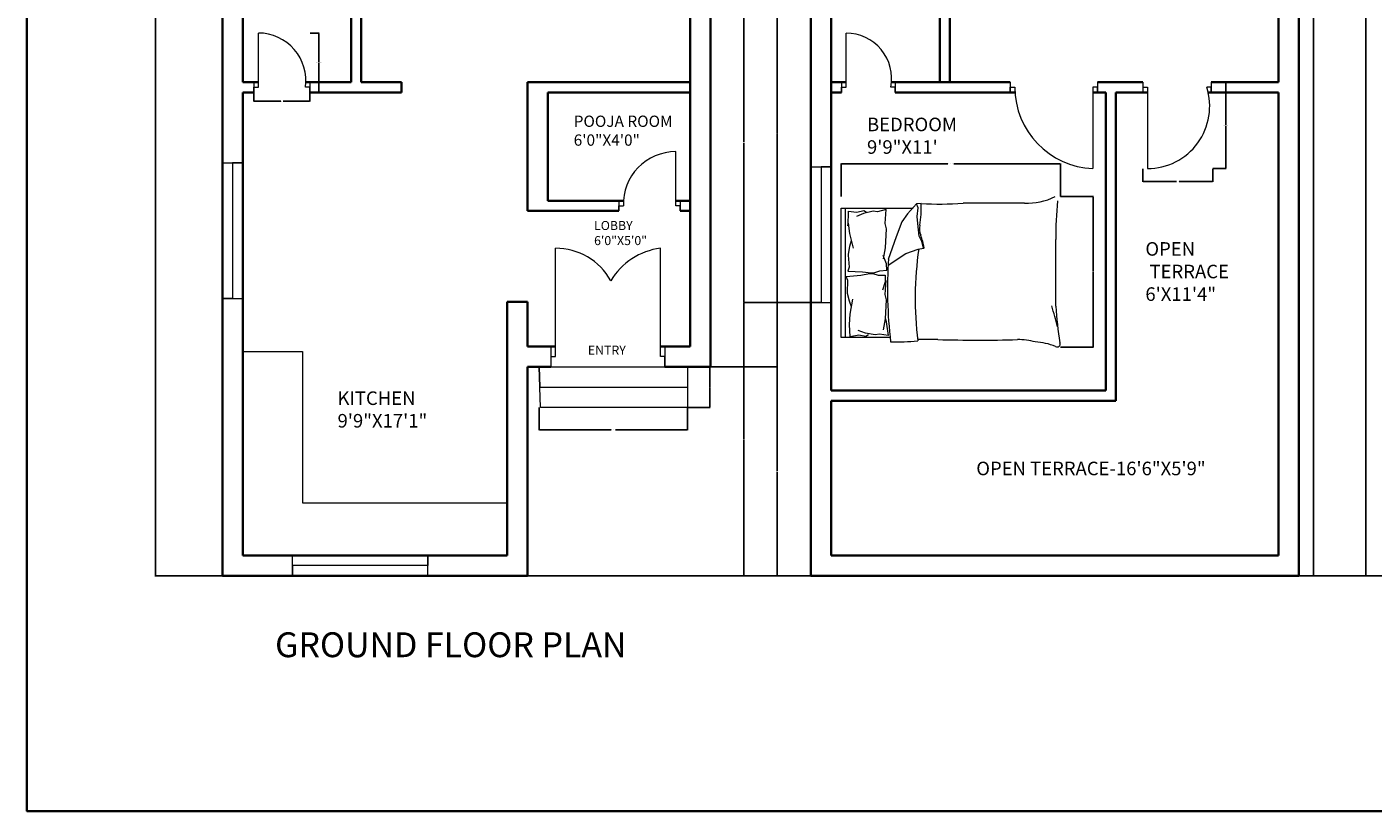
# Model space of a CAD drawing. Units: inches. Extents: x 2003 to 3241, y 1726 to 2849.
# Tile 1 of 7: x 2003 to 2599, y 1726 to 2073. Entities that reach past the tile are written whole.
import ezdxf

# ---------------------------------------------------------------- set-up
doc = ezdxf.new("R2010")
doc.units = ezdxf.units.IN
for name, color, linetype, lineweight in [('A-ANNO-DIMS', 2, 'Continuous', 18), ('A-ANNO-TEXT', 7, 'Continuous', 18), ('A-ANNO-TTLB', 7, 'Continuous', 35), ('A-AREA-IDEN', 7, 'Continuous', 18), ('A-DOOR', 3, 'Continuous', 18), ('A-FLOR-FIXT', 9, 'Continuous', 18), ('A-FLOR-STRS', 7, 'Continuous', 18), ('A-FURN', 8, 'Continuous', 13), ('A-GLAZ', 4, 'Continuous', 18), ('A-WALL', 7, 'Continuous', 35)]:
    doc.layers.add(name, color=color, linetype=linetype, lineweight=lineweight)
doc.styles.get("Standard").update_dxf_attribs({"font": 'arial.ttf'})
doc.dimstyles.get("Standard").update_dxf_attribs({"dimtxt": 0.18, "dimasz": 0.18, "dimexe": 0.18, "dimexo": 0.0625, "dimgap": 0.09, "dimtad": 0, "dimtih": 1, "dimtoh": 1, "dimdec": 4, "dimzin": 0, "dimdsep": 46, "dimtxsty": 'Standard', "dimcen": 0.09, "dimadec": 0, "dimazin": 0, "dimtfac": 1, "dimtdec": 4, "dimtofl": 0, "dimtmove": 0, "dimatfit": 3, "dimfxl": 1, "dimtolj": 1, "dimtzin": 0, "dimarcsym": 0})

# ---------------------------------------------------------------- blocks, each defined once
blk = doc.blocks.new('WIN-60-1')
for p, q in [((0, 60), (9, 60)), ((9, 60), (4.5, 60)), ((4.5, 60), (4.5, 0)), ((4.5, 0), (0, 0)), ((0, 0), (9, 0))]:
    blk.add_line(p, q)
blk = doc.blocks.new('DOOR-ENTRY-PAIR')
for p, q in [((2, 4.5), (2, 52.5)), ((48.48, 4.5), (48.48, 52.5)), ((0, 9), (0, 0)), ((50.48, 9), (50.48, 0)), ((0, 4.5), (2, 4.5)), ((50.48, 4.5), (48.48, 4.5)), ((50.48, 0), (50.48, 4.5))]:
    blk.add_line(p, q)
for centre, radius, start, end in [((2, 24.35), 28.14, 29.23528, 90), ((52.39, 22.67), 30.08, 97.45976, 149.14255)]:
    blk.add_arc(centre, radius, start, end)
blk = doc.blocks.new('DOOR-POOJA')
for p, q in [((25.16, 2.25), (25.16, 26.25)), ((0, 4.5), (0, 0)), ((0, 0), (0, 2.25)), ((0, 2.25), (2, 2.25)), ((27.16, 2.25), (25.16, 2.25)), ((27.16, 4.5), (27.16, 0)), ((27.16, 0), (27.16, 2.25))]:
    blk.add_line(p, q)
blk.add_arc((25.16, 3.08), 23.17, 90, 182.04429)
blk = doc.blocks.new('DOOR-STORE')
for p, q in [((2, 2.25), (2, 26.25)), ((0, 4.5), (0, 0)), ((0, 0), (0, 2.25)), ((0, 2.25), (2, 2.25)), ((24.85, 2.25), (22.85, 2.25)), ((24.85, 4.5), (24.85, 0)), ((24.85, 0), (24.85, 2.25))]:
    blk.add_line(p, q)
blk.add_arc((2, 5.2), 21.05, 351.95387, 90)
blk = doc.blocks.new('DOOR-TERRACE-BEDROOM')
for p, q in [((0, 38.25), (0, 33.75)), ((0, 33.75), (0, 36)), ((0, 36), (2, 36)), ((38.56, 36), (36.56, 36)), ((36.56, 36), (36.56, 0)), ((38.56, 38.25), (38.56, 33.75)), ((38.56, 33.75), (38.56, 36))]:
    blk.add_line(p, q)
blk.add_arc((38.03, 36), 36.03, 180, 267.65676)
blk = doc.blocks.new('DOOR-TERRACE')
for p, q in [((0, 38.25), (0, 33.75)), ((0, 36), (2, 36)), ((2, 36), (2, 0)), ((30.26, 36), (28.26, 36)), ((30.26, 38.25), (30.26, 33.75)), ((30.26, 33.75), (30.26, 36))]:
    blk.add_line(p, q)
blk.add_arc((2, 27.58), 27.58, 270, 17.78542)
blk = doc.blocks.new('STEPS-ENTRY')
for p, q in [((0.54, 0), (0, 18)), ((0, 18), (0.27, 9)), ((5.21, 18), (55.69, 18)), ((55.69, 18), (65.74, 18)), ((65.74, 18), (65.74, 0)), ((0.27, 9), (0.27, 9)), ((0.27, 9), (65.74, 9)), ((65.74, 0), (0.54, 0))]:
    blk.add_line(p, q)
blk = doc.blocks.new('COUNTER-KITCHEN-L')
for p, q in [((0, 67), (26.53, 67)), ((26.53, 67), (26.53, 0)), ((26.53, 0), (117, 0))]:
    blk.add_line(p, q)
blk = doc.blocks.new('BED-DOUBLE')
for p, q in [((4.17, 75.16), (4.17, 96.87)), ((4.17, 96.87), (61.46, 96.87)), ((61.46, 96.87), (61.46, 64.97)), ((4.17, 95.03), (61.46, 95.03)), ((4.67, 92.87), (9.81, 93.27)), ((4.67, 92.9), (5.36, 89.08)), ((6.06, 86.14), (7.27, 89.43)), ((9.81, 93.27), (9.93, 93.24)), ((9.93, 93.24), (14.52, 92.9)), ((14.52, 92.9), (21.1, 91.68)), ((17.81, 92.38), (20.24, 93.24)), ((20.24, 93.24), (23.7, 94.11)), ((23.7, 94.11), (24.09, 94.11)), ((24.09, 94.11), (29.42, 93.94)), ((29.42, 93.94), (31.15, 94.63)), ((31.15, 94.63), (31.84, 88.22)), ((33.54, 93.89), (33.25, 87.44)), ((35.31, 93.3), (33.54, 93.89)), ((40.62, 93.81), (35.31, 93.3)), ((41.01, 93.83), (40.62, 93.81)), ((44.52, 93.18), (41.01, 93.83)), ((50.25, 93.19), (43.75, 91.57)), ((47, 92.47), (44.52, 93.18)), ((54.8, 93.82), (50.25, 93.19)), ((60.08, 93.81), (53.6, 93.92)), ((53.6, 93.92), (54.8, 93.82)), ((59.12, 86.97), (57.7, 90.18)), ((60.08, 93.81), (59.62, 89.96)), ((59.62, 89.96), (60.34, 86.88)), ((5.36, 89.08), (4.84, 85.96)), ((4.84, 85.96), (5.54, 84.75)), ((5.36, 81.8), (6.06, 86.14)), ((31.84, 88.22), (32.54, 84.4)), ((32.54, 84.4), (32.54, 82.84)), ((33.25, 87.44), (32.79, 83.59)), ((32.79, 83.59), (32.89, 82.03)), ((60.08, 82.69), (59.12, 86.97)), ((60.34, 86.88), (59.72, 85.62)), ((5.02, 76.08), (5.71, 79.9)), ((5.71, 79.9), (5.36, 81.8)), ((7.65, 78.14), (12.48, 77.34)), ((20.89, 76.82), (23.24, 77.49)), ((23.24, 77.49), (29.39, 77)), ((28.9, 77.38), (25.13, 78.68)), ((32.54, 82.84), (31.84, 80.59)), ((31.84, 80.59), (31.84, 77.38)), ((32.89, 82.03), (33.72, 79.83)), ((33.72, 79.83), (33.93, 76.62)), ((36.87, 76.8), (40.55, 78.34)), ((39.04, 78.14), (43.87, 77.34)), ((52.28, 76.82), (54.63, 77.49)), ((54.63, 77.49), (60.78, 77)), ((59.85, 80.77), (60.08, 82.69)), ((60.78, 77), (59.85, 80.77)), ((11.13, 76.95), (5.02, 76.08)), ((12.48, 77.34), (11.13, 76.95)), ((12.48, 77.34), (20.89, 76.82)), ((31.84, 77.38), (28.9, 77.38)), ((33.93, 76.62), (36.87, 76.8)), ((36.28, 76.03), (41.3, 68.25)), ((48.73, 72.52), (38.73, 76.03)), ((43.87, 77.34), (52.28, 76.82)), ((55.41, 70.1), (48.73, 72.52)), ((41.3, 68.25), (43.34, 62.87)), ((58.94, 67.51), (55.41, 70.1)), ((63.38, 63.61), (58.94, 67.51)), ((43.34, 62.87), (43.71, 60.45)), ((43.71, 60.45), (46.68, 61.2)), ((46.68, 61.2), (49.1, 62.31)), ((49.1, 62.31), (53.18, 62.87)), ((53.18, 62.87), (57.82, 63.24)), ((57.82, 63.24), (61.54, 62.87)), ((61.54, 62.87), (63.38, 63.61)), ((63.48, 61.52), (63.38, 63.61, 4.64)), ((18.06, 1.87), (47.57, 1.87))]:
    blk.add_line(p, q)
for centre, radius, start, end in [((102.1, 72.78), 99.87, 178.72178, 185.60397), ((25.61, -121.38), 197.77, 86.08655, 96.78213), ((21.29, -90.53), 154.68, 81.78449, 96.90062), ((-200.58, 59.5), 203.94, 358.4762, 1.00819), ((43.92, 60.38), 0.221, 160.24637, 271.13765), ((37.35, 95.1), 35.55, 280.66171, 289.88058), ((52.44, 54.83), 7.46, 78.6608, 113.73842), ((61.53, 104.85), 43.38, 259.87628, 272.56571), ((218.51, 53.34), 155.25, 176.97912, 183.83645), ((581.23, 36.19), 578.22, 178.22771, 181.71854), ((-5405.34, 15.56), 5469.02, 0.00217, 0.28689), ((-32.25, 19.53), 35.53, 346.06484, 358.91125), ((91.3, 14.55), 27.65, 177.47136, 206.46809), ((-25.97, 12.62), 28.25, 337.97508, 356.652), ((1.3, 1.3), 1.31, 146.17358, 293.47814), ((25.69, -143.9), 145.97, 92.99578, 99.40907), ((-20.65, 125.3), 127.63, 283.38322, 287.70533), ((49.34, -157.62), 159.5, 84.4998, 90.63509)]:
    blk.add_arc(centre, radius, start, end)
blk = doc.blocks.new('*D26')
at = {"layer": 'A-ANNO-DIMS', "color": 0, "lineweight": -2, "transparency": 16777216}
for p, q in [((2363.72, 1998.31), (2363.72, 2012.98)), ((2363.9, 2012.8), (2410.85, 2012.8)), ((2460.54, 2012.8), (2413.58, 2012.8)), ((2460.72, 1998.31), (2460.72, 2012.98))]:
    blk.add_line(p, q, dxfattribs=at)
at = {"layer": 'A-ANNO-DIMS', "color": 0, "transparency": 16777216}
for points in [[(2363.9, 2012.83), (2363.9, 2012.77), (2363.72, 2012.8)], [(2460.54, 2012.83), (2460.54, 2012.77), (2460.72, 2012.8)]]:
    blk.add_solid(points, dxfattribs=at)
at = {"layer": 'Defpoints', "color": 0, "transparency": 16777216}
for p in [(2363.72, 2012.8), (2363.72, 1998.25), (2460.72, 1998.25)]:
    blk.add_point(p, dxfattribs=at)
at = {"layer": 'A-ANNO-DIMS', "color": 0, "transparency": 16777216, "insert": (2412.22, 2012.8), "char_height": 0.18, "attachment_point": 5}
blk.add_mtext('\\A1;DOUBLE BED 97 TYP.', dxfattribs=at)
blk = doc.blocks.new('*D27')
at = {"layer": 'A-ANNO-DIMS', "color": 0, "lineweight": -2, "transparency": 16777216}
for p, q in [((2460.78, 1998.25), (2475.44, 1998.25)), ((2475.26, 1998.07), (2475.26, 1965.1)), ((2475.26, 1931.78), (2475.26, 1964.74)), ((2460.78, 1931.6), (2475.44, 1931.6))]:
    blk.add_line(p, q, dxfattribs=at)
at = {"layer": 'A-ANNO-DIMS', "color": 0, "transparency": 16777216}
for points in [[(2475.23, 1998.07), (2475.29, 1998.07), (2475.26, 1998.25)], [(2475.23, 1931.78), (2475.29, 1931.78), (2475.26, 1931.6)]]:
    blk.add_solid(points, dxfattribs=at)
at = {"layer": 'Defpoints', "color": 0, "transparency": 16777216}
for p in [(2460.72, 1998.25), (2475.26, 1998.25), (2460.72, 1931.6)]:
    blk.add_point(p, dxfattribs=at)
at = {"layer": 'A-ANNO-DIMS', "color": 0, "transparency": 16777216, "insert": (2475.26, 1964.92), "char_height": 0.18, "attachment_point": 5}
blk.add_mtext('\\A1;67 TYP.', dxfattribs=at)
blk = doc.blocks.new('*D40')
at = {"layer": 'A-ANNO-DIMS', "color": 0, "lineweight": -2, "transparency": 16777216}
for p, q in [((2128.61, 2070.66), (2132.66, 2070.66)), ((2132.48, 2070.48), (2132.48, 2057.72)), ((2132.48, 2044.59), (2132.48, 2057.36)), ((2128.61, 2044.41), (2132.66, 2044.41))]:
    blk.add_line(p, q, dxfattribs=at)
at = {"layer": 'A-ANNO-DIMS', "color": 0, "transparency": 16777216}
for points in [[(2132.45, 2070.48), (2132.51, 2070.48), (2132.48, 2070.66)], [(2132.45, 2044.59), (2132.51, 2044.59), (2132.48, 2044.41)]]:
    blk.add_solid(points, dxfattribs=at)
at = {"layer": 'Defpoints', "color": 0, "transparency": 16777216}
for p in [(2128.55, 2070.66), (2132.48, 2070.66), (2128.55, 2044.41)]:
    blk.add_point(p, dxfattribs=at)
at = {"layer": 'A-ANNO-DIMS', "color": 0, "transparency": 16777216, "insert": (2132.48, 2057.54), "char_height": 0.18, "attachment_point": 5}
blk.add_mtext('\\A1;STORE DOOR 26 TYP.', dxfattribs=at)
blk = doc.blocks.new('*D41')
at = {"layer": 'A-ANNO-DIMS', "color": 0, "lineweight": -2, "transparency": 16777216}
for p, q in [((2103.7, 2044.35), (2103.7, 2040.3)), ((2128.55, 2044.35), (2128.55, 2040.3)), ((2103.88, 2040.48), (2115.59, 2040.48)), ((2128.37, 2040.48), (2116.65, 2040.48))]:
    blk.add_line(p, q, dxfattribs=at)
at = {"layer": 'A-ANNO-DIMS', "color": 0, "transparency": 16777216}
for points in [[(2103.88, 2040.51), (2103.88, 2040.45), (2103.7, 2040.48)], [(2128.37, 2040.51), (2128.37, 2040.45), (2128.55, 2040.48)]]:
    blk.add_solid(points, dxfattribs=at)
at = {"layer": 'Defpoints', "color": 0, "transparency": 16777216}
for p in [(2103.7, 2044.41), (2128.55, 2044.41), (2128.55, 2040.48)]:
    blk.add_point(p, dxfattribs=at)
at = {"layer": 'A-ANNO-DIMS', "color": 0, "transparency": 16777216, "insert": (2116.12, 2040.48), "char_height": 0.18, "attachment_point": 5}
blk.add_mtext('\\A1;25 TYP.', dxfattribs=at)
blk = doc.blocks.new('*D50')
at = {"layer": 'A-ANNO-DIMS', "color": 0, "lineweight": -2, "transparency": 16777216}
for p, q in [((2528.24, 2048.91), (2534.1, 2048.91)), ((2533.92, 2048.73), (2533.92, 2029.97)), ((2533.92, 2010.84), (2533.92, 2029.61)), ((2528.24, 2010.66), (2534.1, 2010.66))]:
    blk.add_line(p, q, dxfattribs=at)
at = {"layer": 'A-ANNO-DIMS', "color": 0, "transparency": 16777216}
for points in [[(2533.89, 2048.73), (2533.95, 2048.73), (2533.92, 2048.91)], [(2533.89, 2010.84), (2533.95, 2010.84), (2533.92, 2010.66)]]:
    blk.add_solid(points, dxfattribs=at)
at = {"layer": 'Defpoints', "color": 0, "transparency": 16777216}
for p in [(2528.18, 2048.91), (2533.92, 2048.91), (2528.18, 2010.66)]:
    blk.add_point(p, dxfattribs=at)
at = {"layer": 'A-ANNO-DIMS', "color": 0, "transparency": 16777216, "insert": (2533.92, 2029.79), "char_height": 0.18, "attachment_point": 5}
blk.add_mtext('\\A1;TERRACE DOOR 38 TYP.', dxfattribs=at)
blk = doc.blocks.new('*D51')
at = {"layer": 'A-ANNO-DIMS', "color": 0, "lineweight": -2, "transparency": 16777216}
for p, q in [((2497.23, 2010.6), (2497.23, 2004.75)), ((2528.18, 2010.6), (2528.18, 2004.75)), ((2497.41, 2004.93), (2512.18, 2004.93)), ((2528, 2004.93), (2513.23, 2004.93))]:
    blk.add_line(p, q, dxfattribs=at)
at = {"layer": 'A-ANNO-DIMS', "color": 0, "transparency": 16777216}
for points in [[(2497.41, 2004.96), (2497.41, 2004.9), (2497.23, 2004.93)], [(2528, 2004.96), (2528, 2004.9), (2528.18, 2004.93)]]:
    blk.add_solid(points, dxfattribs=at)
at = {"layer": 'Defpoints', "color": 0, "transparency": 16777216}
for p in [(2497.23, 2010.66), (2528.18, 2010.66), (2528.18, 2004.93)]:
    blk.add_point(p, dxfattribs=at)
at = {"layer": 'A-ANNO-DIMS', "color": 0, "transparency": 16777216, "insert": (2512.71, 2004.93), "char_height": 0.18, "attachment_point": 5}
blk.add_mtext('\\A1;31 TYP.', dxfattribs=at)
blk = doc.blocks.new('*D56')
at = {"layer": 'A-ANNO-DIMS', "color": 0, "lineweight": -2, "transparency": 16777216}
for p, q in [((2229.98, 1904.85), (2229.98, 1894.87)), ((2295.72, 1904.85), (2295.72, 1894.87)), ((2230.16, 1895.05), (2261.88, 1895.05)), ((2295.54, 1895.05), (2263.83, 1895.05))]:
    blk.add_line(p, q, dxfattribs=at)
at = {"layer": 'A-ANNO-DIMS', "color": 0, "transparency": 16777216}
for points in [[(2230.16, 1895.08), (2230.16, 1895.02), (2229.98, 1895.05)], [(2295.54, 1895.08), (2295.54, 1895.02), (2295.72, 1895.05)]]:
    blk.add_solid(points, dxfattribs=at)
at = {"layer": 'Defpoints', "color": 0, "transparency": 16777216}
for p in [(2229.98, 1904.91), (2295.72, 1904.91), (2295.72, 1895.05)]:
    blk.add_point(p, dxfattribs=at)
at = {"layer": 'A-ANNO-DIMS', "color": 0, "transparency": 16777216, "insert": (2262.85, 1895.05), "char_height": 0.18, "attachment_point": 5}
blk.add_mtext('\\A1;STEPS 66 TYP.', dxfattribs=at)
blk = doc.blocks.new('*D57')
at = {"layer": 'A-ANNO-DIMS', "color": 0, "lineweight": -2, "transparency": 16777216}
for p, q in [((2295.79, 1922.91), (2305.77, 1922.91)), ((2305.59, 1922.73), (2305.59, 1914.1)), ((2305.59, 1905.09), (2305.59, 1913.73)), ((2295.79, 1904.91), (2305.77, 1904.91))]:
    blk.add_line(p, q, dxfattribs=at)
at = {"layer": 'A-ANNO-DIMS', "color": 0, "transparency": 16777216}
for points in [[(2305.56, 1922.73), (2305.62, 1922.73), (2305.59, 1922.91)], [(2305.56, 1905.09), (2305.62, 1905.09), (2305.59, 1904.91)]]:
    blk.add_solid(points, dxfattribs=at)
at = {"layer": 'Defpoints', "color": 0, "transparency": 16777216}
for p in [(2295.72, 1922.91), (2305.59, 1922.91), (2295.72, 1904.91)]:
    blk.add_point(p, dxfattribs=at)
at = {"layer": 'A-ANNO-DIMS', "color": 0, "transparency": 16777216, "insert": (2305.59, 1913.91), "char_height": 0.18, "attachment_point": 5}
blk.add_mtext('\\A1;18 TYP.', dxfattribs=at)
blk = doc.blocks.new('*D65')
at = {"layer": 'A-ANNO-DIMS', "color": 0, "lineweight": -2, "transparency": 16777216}
for p, q in [((2089.72, 2369.91), (2059.95, 2369.91)), ((2060.13, 2369.73), (2060.13, 2100.35)), ((2060.13, 1830.59), (2060.13, 2099.98)), ((2089.72, 1830.41), (2059.95, 1830.41))]:
    blk.add_line(p, q, dxfattribs=at)
at = {"layer": 'A-ANNO-DIMS', "color": 0, "transparency": 16777216}
for points in [[(2060.1, 2369.73), (2060.16, 2369.73), (2060.13, 2369.91)], [(2060.1, 1830.59), (2060.16, 1830.59), (2060.13, 1830.41)]]:
    blk.add_solid(points, dxfattribs=at)
at = {"layer": 'Defpoints', "color": 0, "transparency": 16777216}
for p in [(2060.13, 2369.91), (2089.78, 2369.91), (2089.78, 1830.41)]:
    blk.add_point(p, dxfattribs=at)
at = {"layer": 'A-ANNO-DIMS', "color": 0, "transparency": 16777216, "insert": (2060.13, 2100.16), "char_height": 0.18, "attachment_point": 5}
blk.add_mtext('\\A1;539.5', dxfattribs=at)
blk = doc.blocks.new('*D66')
at = {"layer": 'A-ANNO-DIMS', "color": 0, "lineweight": -2, "transparency": 16777216}
for p, q in [((2305.84, 1922.91), (2335.61, 1922.91)), ((2335.43, 1922.73), (2335.43, 1876.85)), ((2335.43, 1830.59), (2335.43, 1876.48)), ((2224.84, 1830.41), (2335.61, 1830.41))]:
    blk.add_line(p, q, dxfattribs=at)
at = {"layer": 'A-ANNO-DIMS', "color": 0, "transparency": 16777216}
for points in [[(2335.4, 1922.73), (2335.46, 1922.73), (2335.43, 1922.91)], [(2335.4, 1830.59), (2335.46, 1830.59), (2335.43, 1830.41)]]:
    blk.add_solid(points, dxfattribs=at)
at = {"layer": 'Defpoints', "color": 0, "transparency": 16777216}
for p in [(2305.78, 1922.91), (2335.43, 1922.91), (2224.78, 1830.41)]:
    blk.add_point(p, dxfattribs=at)
at = {"layer": 'A-ANNO-DIMS', "color": 0, "transparency": 16777216, "insert": (2335.43, 1876.66), "char_height": 0.18, "attachment_point": 5}
blk.add_mtext('\\A1;92.5', dxfattribs=at)
blk = doc.blocks.new('*D67')
at = {"layer": 'A-ANNO-DIMS', "color": 0, "lineweight": -2, "transparency": 16777216}
for p, q in [((2305.84, 2129.81), (2335.61, 2129.81)), ((2335.43, 2129.63), (2335.43, 2026.55)), ((2335.43, 1923.09), (2335.43, 2026.18)), ((2305.84, 1922.91), (2335.61, 1922.91))]:
    blk.add_line(p, q, dxfattribs=at)
at = {"layer": 'A-ANNO-DIMS', "color": 0, "transparency": 16777216}
for points in [[(2335.4, 2129.63), (2335.46, 2129.63), (2335.43, 2129.81)], [(2335.4, 1923.09), (2335.46, 1923.09), (2335.43, 1922.91)]]:
    blk.add_solid(points, dxfattribs=at)
at = {"layer": 'Defpoints', "color": 0, "transparency": 16777216}
for p in [(2305.78, 2129.81), (2335.43, 2129.81), (2305.78, 1922.91)]:
    blk.add_point(p, dxfattribs=at)
at = {"layer": 'A-ANNO-DIMS', "color": 0, "transparency": 16777216, "insert": (2335.43, 2026.36), "char_height": 0.18, "attachment_point": 5}
blk.add_mtext('\\A1;206.9', dxfattribs=at)
blk = doc.blocks.new('*D71')
at = {"layer": 'A-ANNO-DIMS', "color": 0, "lineweight": -2, "transparency": 16777216}
for p, q in [((2566.36, 2369.91), (2596.13, 2369.91)), ((2595.95, 2369.73), (2595.95, 2100.35)), ((2595.95, 1830.59), (2595.95, 2099.98)), ((2566.36, 1830.41), (2596.13, 1830.41))]:
    blk.add_line(p, q, dxfattribs=at)
at = {"layer": 'A-ANNO-DIMS', "color": 0, "transparency": 16777216}
for points in [[(2595.92, 2369.73), (2595.98, 2369.73), (2595.95, 2369.91)], [(2595.92, 1830.59), (2595.98, 1830.59), (2595.95, 1830.41)]]:
    blk.add_solid(points, dxfattribs=at)
at = {"layer": 'Defpoints', "color": 0, "transparency": 16777216}
for p in [(2566.3, 2369.91), (2595.95, 2369.91), (2566.3, 1830.41)]:
    blk.add_point(p, dxfattribs=at)
at = {"layer": 'A-ANNO-DIMS', "color": 0, "transparency": 16777216, "insert": (2595.95, 2100.16), "char_height": 0.18, "attachment_point": 5}
blk.add_mtext('\\A1;539.5', dxfattribs=at)
blk = doc.blocks.new('*D72')
at = {"layer": 'A-ANNO-DIMS', "color": 0, "lineweight": -2, "transparency": 16777216}
for p, q in [((2350.24, 1951.42), (2320.47, 1951.42)), ((2320.65, 1951.24), (2320.65, 1891.09)), ((2320.65, 1830.59), (2320.65, 1890.73)), ((2350.24, 1830.41), (2320.47, 1830.41))]:
    blk.add_line(p, q, dxfattribs=at)
at = {"layer": 'A-ANNO-DIMS', "color": 0, "transparency": 16777216}
for points in [[(2320.62, 1951.24), (2320.68, 1951.24), (2320.65, 1951.42)], [(2320.62, 1830.59), (2320.68, 1830.59), (2320.65, 1830.41)]]:
    blk.add_solid(points, dxfattribs=at)
at = {"layer": 'Defpoints', "color": 0, "transparency": 16777216}
for p in [(2320.65, 1951.42), (2350.3, 1951.42), (2350.3, 1830.41)]:
    blk.add_point(p, dxfattribs=at)
at = {"layer": 'A-ANNO-DIMS', "color": 0, "transparency": 16777216, "insert": (2320.65, 1890.91), "char_height": 0.18, "attachment_point": 5}
blk.add_mtext('\\A1;121', dxfattribs=at)
blk = doc.blocks.new('*D73')
at = {"layer": 'A-ANNO-DIMS', "color": 0, "lineweight": -2, "transparency": 16777216}
for p, q in [((2350.24, 2092.82), (2320.47, 2092.82)), ((2320.65, 2092.64), (2320.65, 2022.3)), ((2320.65, 1951.6), (2320.65, 2021.94)), ((2350.24, 1951.42), (2320.47, 1951.42))]:
    blk.add_line(p, q, dxfattribs=at)
at = {"layer": 'A-ANNO-DIMS', "color": 0, "transparency": 16777216}
for points in [[(2320.62, 2092.64), (2320.68, 2092.64), (2320.65, 2092.82)], [(2320.62, 1951.6), (2320.68, 1951.6), (2320.65, 1951.42)]]:
    blk.add_solid(points, dxfattribs=at)
at = {"layer": 'Defpoints', "color": 0, "transparency": 16777216}
for p in [(2320.65, 2092.82), (2350.3, 2092.82), (2350.3, 1951.42)]:
    blk.add_point(p, dxfattribs=at)
at = {"layer": 'A-ANNO-DIMS', "color": 0, "transparency": 16777216, "insert": (2320.65, 2022.12), "char_height": 0.18, "attachment_point": 5}
blk.add_mtext('\\A1;141.4', dxfattribs=at)
blk = doc.blocks.new('*D77')
at = {"layer": 'A-ANNO-DIMS', "color": 0, "lineweight": -2, "transparency": 16777216}
for p, q in [((2632.38, 2369.91), (2572.63, 2369.91)), ((2572.81, 2369.73), (2572.81, 2100.35)), ((2572.81, 1830.59), (2572.81, 2099.98)), ((2632.38, 1830.41), (2572.63, 1830.41))]:
    blk.add_line(p, q, dxfattribs=at)
at = {"layer": 'A-ANNO-DIMS', "color": 0, "transparency": 16777216}
for points in [[(2572.78, 2369.73), (2572.84, 2369.73), (2572.81, 2369.91)], [(2572.78, 1830.59), (2572.84, 1830.59), (2572.81, 1830.41)]]:
    blk.add_solid(points, dxfattribs=at)
at = {"layer": 'Defpoints', "color": 0, "transparency": 16777216}
for p in [(2572.81, 2369.91), (2632.44, 2369.91), (2632.44, 1830.41)]:
    blk.add_point(p, dxfattribs=at)
at = {"layer": 'A-ANNO-DIMS', "color": 0, "transparency": 16777216, "insert": (2572.81, 2100.16), "char_height": 0.18, "attachment_point": 5}
blk.add_mtext('\\A1;539.5', dxfattribs=at)

msp = doc.modelspace()

# ---------------------------------------------------------------- linework, layer by layer
at = {"layer": 'A-ANNO-TTLB'}
msp.add_lwpolyline([(2003.2633, 2848.7261), (3241.1194, 2848.7261), (3241.1194, 1726.227), (2003.2633, 1726.227)], close=True, dxfattribs=at)
at = {"layer": 'A-DOOR'}
for p, q in [((2365.8505, 2046.6635), (2365.8505, 2070.6635)), ((2363.8505, 2048.9135), (2363.8505, 2044.4135)), ((2363.8505, 2044.4135), (2363.8505, 2046.6635)), ((2363.8505, 2046.6635), (2365.8505, 2046.6635)), ((2387.622, 2046.6635), (2385.622, 2046.6635)), ((2387.622, 2048.9135), (2387.622, 2044.4135)), ((2387.622, 2044.4135), (2387.622, 2046.6635))]:
    msp.add_line(p, q, dxfattribs=at)
msp.add_arc((2365.8505, 2050.5196), 20.1439, 348.9640184, 90, dxfattribs=at)
at = {"layer": 'A-WALL'}
for p, q in [((2089.7784, 2369.9135), (2089.7784, 1830.4135)), ((2305.7784, 2369.9135), (2305.7784, 1922.9135)), ((2350.3008, 2369.9135), (2350.3008, 1836.4016)), ((2566.3008, 2369.9135), (2566.3008, 1836.4016)), ((2557.3008, 2360.9135), (2557.3008, 2048.9135)), ((2151.2784, 2224.4135), (2151.2784, 2048.9135)), ((2296.7784, 2224.4135), (2296.7784, 1931.9135)), ((2359.3008, 2224.4135), (2359.3008, 1912.4135)), ((2411.8008, 2048.9135), (2411.8008, 2224.4135)), ((2098.7784, 2135.9135), (2098.7784, 2048.9135)), ((2146.7784, 2135.9135), (2146.7784, 2048.9135)), ((2407.3008, 2135.9135), (2407.3008, 2048.9135)), ((2098.7784, 2048.9135), (2105.7015, 2048.9135)), ((2098.7784, 2044.4135), (2103.7015, 2044.4135)), ((2098.7784, 2044.4135), (2098.7784, 1839.4135)), ((2126.7431, 2048.9135), (2146.7784, 2048.9135)), ((2128.5474, 2044.4135), (2151.2784, 2044.4135)), ((2151.2784, 2048.9135), (2169.1304, 2048.9135)), ((2151.2784, 2044.4135), (2169.1304, 2044.4135)), ((2169.1304, 2048.9135), (2169.1304, 2044.4135)), ((2224.7784, 2044.4135), (2224.7784, 2048.9135)), ((2224.7784, 2048.9135), (2296.7784, 2048.9135)), ((2224.7784, 2044.4135), (2224.7784, 1991.9135)), ((2296.7784, 2044.4135), (2233.7784, 2044.4135)), ((2233.7784, 1996.4135), (2233.7784, 2044.4135)), ((2233.7784, 2044.4135), (2296.7784, 2044.4135)), ((2359.3008, 2048.9135), (2365.8505, 2048.9135)), ((2359.3008, 2044.4135), (2363.8505, 2044.4135)), ((2359.3008, 2044.4135), (2363.8505, 2044.4135)), ((2385.9304, 2048.9135), (2438.5561, 2048.9135)), ((2387.622, 2044.4135), (2440.6264, 2044.4135)), ((2387.622, 2044.4135), (2411.8008, 2044.4135)), ((2475.1131, 2044.4135), (2480.8008, 2044.4135)), ((2477.1131, 2048.9135), (2497.2319, 2048.9135)), ((2480.8008, 1912.4135), (2480.8008, 2044.4135)), ((2485.3008, 2044.4135), (2485.3008, 1907.9135)), ((2485.3008, 2044.4135), (2499.2319, 2044.4135)), ((2499.2319, 2044.4135), (2485.3008, 2044.4135)), ((2557.3008, 2044.4135), (2526.1087, 2044.4135)), ((2526.1087, 2044.4135), (2557.3008, 2044.4135)), ((2527.4906, 2048.9135), (2557.3008, 2048.9135)), ((2557.3008, 2044.4135), (2557.3008, 1839.4135)), ((2233.7784, 1996.4135), (2267.3074, 1996.4135)), ((2290.437, 1996.4135), (2296.7784, 1996.4135)), ((2224.7784, 1991.9135), (2265.2784, 1991.9135)), ((2224.7784, 1991.9135), (2233.7784, 1991.9135)), ((2292.437, 1991.9135), (2296.7784, 1991.9135)), ((2215.7784, 1931.9135), (2215.7784, 1951.6161)), ((2215.7784, 1951.6161), (2224.7784, 1951.6161)), ((2224.7784, 1951.6161), (2224.7784, 1931.9135)), ((2215.7784, 1839.4135), (2215.7784, 1931.9135)), ((2224.7784, 1931.9135), (2237.1913, 1931.9135)), ((2283.6705, 1931.9135), (2296.7784, 1931.9135)), ((2224.7784, 1922.9135), (2235.1913, 1922.9135)), ((2224.7784, 1922.9135), (2224.7784, 1839.4135)), ((2285.6705, 1922.9135), (2305.7784, 1922.9135)), ((2359.3008, 1912.4135), (2480.8008, 1912.4135)), ((2359.3008, 1907.9135), (2485.3008, 1907.9135)), ((2359.3008, 1907.9135), (2359.3008, 1839.4135)), ((2485.3008, 1907.9135), (2480.8008, 1907.9135)), ((2098.7784, 1839.4135), (2215.7784, 1839.4135)), ((2098.7784, 1839.4135), (2215.7784, 1839.4135)), ((2224.7784, 1839.4135), (2224.7784, 1830.4135)), ((2350.3008, 1830.4135), (2350.3008, 1836.4016)), ((2359.3008, 1839.4135), (2557.3008, 1839.4135)), ((2566.3008, 1839.4135), (2566.3008, 1830.4135)), ((2089.7784, 1830.4135), (2224.7784, 1830.4135)), ((2566.3008, 1830.4135), (2350.3008, 1830.4135))]:
    msp.add_line(p, q, dxfattribs=at)

# ---------------------------------------------------------------- block references
at = {"layer": 'A-DOOR'}
for name, p in [('DOOR-STORE', (2103.701, 2044.414)), ('DOOR-TERRACE-BEDROOM', (2438.556, 2010.664)), ('DOOR-TERRACE', (2497.232, 2010.664)), ('DOOR-POOJA', (2265.278, 1991.914)), ('DOOR-ENTRY-PAIR', (2235.191, 1922.914))]:
    msp.add_blockref(name, p, dxfattribs=at)
at = {"layer": 'A-FLOR-FIXT'}
msp.add_blockref('COUNTER-KITCHEN-L', (2098.778, 1862.743), dxfattribs=at)
at = {"layer": 'A-FLOR-STRS'}
msp.add_blockref('STEPS-ENTRY', (2229.985, 1904.914), dxfattribs=at)
at = {"layer": 'A-FURN', "rotation": 90}
msp.add_blockref('BED-DOUBLE', (2460.5888, 1931.698), dxfattribs=at)
at = {"layer": 'A-GLAZ'}
for p in [(2089.778, 1953.19), (2350.3004, 1951.4154)]:
    msp.add_blockref('WIN-60-1', p, dxfattribs=at)
at = {"layer": 'A-GLAZ', "extrusion": (0, 0, -1), "zscale": -1, "rotation": 90}
msp.add_blockref('WIN-60-1', (-2120.7796, 1830.4131), dxfattribs=at)

# ---------------------------------------------------------------- texts
at = {"layer": 'A-ANNO-TEXT', "insert": (2113.0973, 1805.354), "char_height": 11, "attachment_point": 1}
msp.add_mtext_dynamic_manual_height_columns('GROUND FLOOR PLAN', width=206.837792, gutter_width=12.5, heights=[0], dxfattribs=at)
at = {"layer": 'A-AREA-IDEN', "attachment_point": 1}
for s, width, insert, char_height in [('POOJA ROOM\\P6\'0"X4\'0"', 98.120857, (2245.2905, 2034.1144), 5), ('BEDROOM\\P9\'9"X11\'', 99.989555, (2375.1235, 2033.2029), 6), ('LOBBY\\P6\'0"X5\'0"', 82.349771, (2254.3147, 1987.4629), 4), ('OPEN\\P TERRACE\\P6\'X11\'4"', 115.234266, (2498.3464, 1978.1016), 6), ('ENTRY', 32.095586, (2251.5749, 1932.274), 4), ('KITCHEN\\P9\'9"X17\'1"', 47.571551, (2140.7589, 1912.0195), 6), ('OPEN TERRACE-16\'6"X5\'9"', 104.137504, (2423.4894, 1880.9065), 6)]:
    msp.add_mtext_dynamic_manual_height_columns(s, width=width, gutter_width=12.5, heights=[0], dxfattribs=dict(at, insert=insert, char_height=char_height))

# ---------------------------------------------------------------- dimensions: what is measured, and where the dimension line sits
at = {"layer": 'A-ANNO-DIMS'}
for base, p1, p2, override, picture, middle in [((2060.1284, 2369.9135), (2089.7784, 1830.4135), (2089.7784, 2369.9135), {"dimdec": 1, "dimlfac": 1, "dimrnd": 0, "dimzin": 0, "dimdsep": 46, "dimlunit": 2}, '*D65', (2060.1284, 2100.1635)), ((2595.9508, 2369.9135), (2566.3008, 1830.4135), (2566.3008, 2369.9135), {"dimdec": 1, "dimlfac": 1, "dimrnd": 0, "dimzin": 0, "dimdsep": 46, "dimlunit": 2}, '*D71', (2595.9508, 2100.1635)), ((2572.8116, 2369.9135), (2632.4427, 1830.4135), (2632.4427, 2369.9135), {"dimdec": 1, "dimlfac": 1, "dimrnd": 0, "dimzin": 0, "dimdsep": 46, "dimlunit": 2}, '*D77', (2572.8116, 2100.1635)), ((2335.4284, 2129.8149), (2305.7784, 1922.9135), (2305.7784, 2129.8149), {"dimdec": 1, "dimlfac": 1, "dimrnd": 0, "dimzin": 0, "dimdsep": 46, "dimlunit": 2}, '*D67', (2335.4284, 2026.3642)), ((2320.6508, 2092.8234), (2350.3008, 1951.4156), (2350.3008, 2092.8234), {"dimdec": 1, "dimlfac": 1, "dimrnd": 0, "dimzin": 0, "dimdsep": 46, "dimlunit": 2}, '*D73', (2320.6508, 2022.1195)), ((2320.6508, 1951.4156), (2350.3008, 1830.4135), (2350.3008, 1951.4156), {"dimdec": 0, "dimlfac": 1, "dimrnd": 0, "dimzin": 0, "dimdsep": 46, "dimlunit": 2}, '*D72', (2320.6508, 1890.9146)), ((2335.4284, 1922.9135), (2224.7784, 1830.4135), (2305.7784, 1922.9135), {"dimdec": 1, "dimlfac": 1, "dimrnd": 0, "dimzin": 0, "dimdsep": 46, "dimlunit": 2}, '*D66', (2335.4284, 1876.6635))]:
    dim = msp.add_linear_dim(base=base, p1=p1, p2=p2, angle=90, dimstyle='Standard', override=override, dxfattribs=at)
    dim.commit()
    dim.dimension.update_dxf_attribs({"geometry": picture, "text_midpoint": middle})
for base, p1, p2, angle, text, picture, middle in [((2132.4849, 2070.6635), (2128.5474, 2044.4135), (2128.5474, 2070.6635), 90, 'STORE DOOR <> TYP.', '*D40', (2132.4849, 2057.5385)), ((2533.9189, 2048.9135), (2528.1814, 2010.6635), (2528.1814, 2048.9135), 90, 'TERRACE DOOR <> TYP.', '*D50', (2533.9189, 2029.7885)), ((2363.7164, 2012.7964), (2460.7151, 1998.2466), (2363.7164, 1998.2466), 180, 'DOUBLE BED <> TYP.', '*D26', (2412.2158, 2012.7964)), ((2475.265, 1998.2466), (2460.7151, 1931.5951), (2460.7151, 1998.2466), 90, '<> TYP.', '*D27', (2475.265, 1964.9208)), ((2305.5854, 1922.9135), (2295.7244, 1904.9135), (2295.7244, 1922.9135), 90, '<> TYP.', '*D57', (2305.5854, 1913.9135))]:
    dim = msp.add_linear_dim(base=base, p1=p1, p2=p2, angle=angle, text=text, dimstyle='Standard', override={"dimdec": 0, "dimlfac": 1, "dimrnd": 0, "dimzin": 0, "dimdsep": 46, "dimlunit": 2}, dxfattribs=at)
    dim.commit()
    dim.dimension.update_dxf_attribs({"geometry": picture, "text_midpoint": middle})
for base, p1, p2, text, picture, middle in [((2128.5474, 2040.476), (2103.7015, 2044.4135), (2128.5474, 2044.4135), '<> TYP.', '*D41', (2116.1244, 2040.476)), ((2528.1814, 2004.926), (2497.2319, 2010.6635), (2528.1814, 2010.6635), '<> TYP.', '*D51', (2512.7067, 2004.926)), ((2295.7244, 1895.0526), (2229.9849, 1904.9135), (2295.7244, 1904.9135), 'STEPS <> TYP.', '*D56', (2262.8546, 1895.0526))]:
    dim = msp.add_linear_dim(base=base, p1=p1, p2=p2, text=text, dimstyle='Standard', override={"dimdec": 0, "dimlfac": 1, "dimrnd": 0, "dimzin": 0, "dimdsep": 46, "dimlunit": 2}, dxfattribs=at)
    dim.commit()
    dim.dimension.update_dxf_attribs({"geometry": picture, "text_midpoint": middle})

doc.saveas('drawing.dxf')
